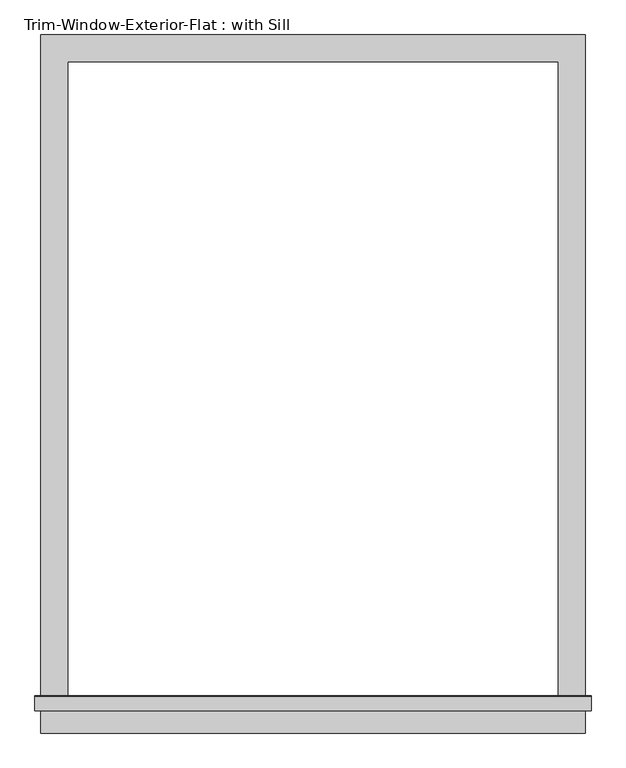
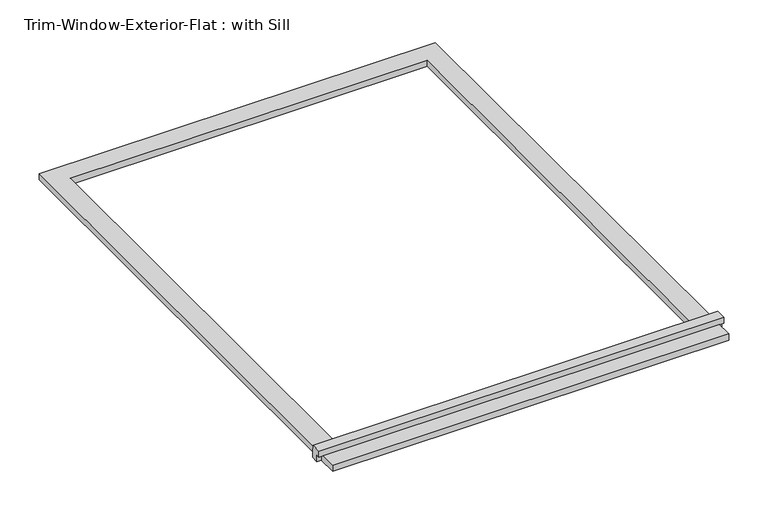
"""IFC4 building model written with IfcOpenShell, lengths in millimetres: proxy geometry, Trim-Window-Exterior-Flat : with Sill."""

from ifc_helpers import new_model, si_unit, frame, origin, origin_with_axes, place, context, project, spatial, polyline, outline, extrude, source, transform, mapped, element, save


def trim_window_exterior_flat_with_sill_4930676f(model_context):
    return source(origin(), model_context, "Body", "SweptSolid", [
        extrude(outline(polyline([(577.85, -1368.3823709), (577.85, -1425.5323709), (-577.85, -1425.5323709), (-577.85, -1368.3823709), (577.85, -1368.3823709)])), origin_with_axes(), (0.0, 0.0, 1.0), 19.05),
        extrude(outline(polyline([(-1377.95, 38.1), (-1348.6580645, 38.1), (-1346.2, 19.05), (-1346.2, 0.0), (-1368.3823709, 0.0), (-1368.3823709, 19.05), (-1377.95, 19.05), (-1377.95, 38.1)])), frame((-590.55, 0.0, 0.0), z_axis=(1.0, 0.0, 0.0), x_axis=(0.0, 1.0, 0.0)), (0.0, 0.0, 1.0), 1181.1),
        extrude(outline(polyline([(-577.85, 57.15), (577.85, 57.15), (577.85, -1346.2), (520.7, -1346.2), (520.7, 0.0), (-520.7, 0.0), (-520.7, -1346.2), (-577.85, -1346.2), (-577.85, 57.15)])), origin_with_axes(), (0.0, 0.0, 1.0), 19.05),
    ])


if __name__ == "__main__":
    model = new_model("IFC4")
    model_context = context("Model", 3, world=origin())
    ifc_project = project(units=[si_unit("LENGTHUNIT", "METRE", prefix="MILLI")], contexts=[model_context])
    site = spatial("IfcSite", under=ifc_project)
    building = spatial("IfcBuilding", under=site)
    placement = place(None, origin())
    trim_window_exterior_flat_with_sill_shape = trim_window_exterior_flat_with_sill_4930676f(model_context)
    element("IfcBuildingElementProxy", 1, Name="Trim-Window-Exterior-Flat : with Sill", ObjectType="Trim-Window-Exterior-Flat : with Sill", at=placement, inside=building, context=model_context, shape_type="MappedRepresentation", body=[
        mapped(trim_window_exterior_flat_with_sill_shape, transform((0.0, 0.0, 0.0), x_axis=(1.0, 0.0, 0.0), y_axis=(0.0, 1.0, 0.0), z_axis=(0.0, 0.0, 1.0))),
    ])
    save(model, "model.ifc")

# Revit data of these elements
# Type "Trim-Window-Exterior-Flat : with Sill"
#   Trim Width = 0' - 2 1/4"
#   Trim Thickness_Picture Frame = 0' - 1 1/4"
#   Trim Thickness_with Sill = 0' - 0 3/4"
#   Sill Thickness = 0' - 1 1/4"
#   Opening Width [instance default] = 2' - 0"
#   Opening Height [instance default] = 3' - 0"
#   Default Elevation = 4' - 0"
#   Sill = yes
#   Picture Frame = no
#   Trim Material [instance default] = none
# Element 1 (IfcBuildingElementProxy, "Trim-Window-Exterior-Flat : with Sill")
#   Opening Width = 3' - 5"
#   Opening Height = 4' - 5"
